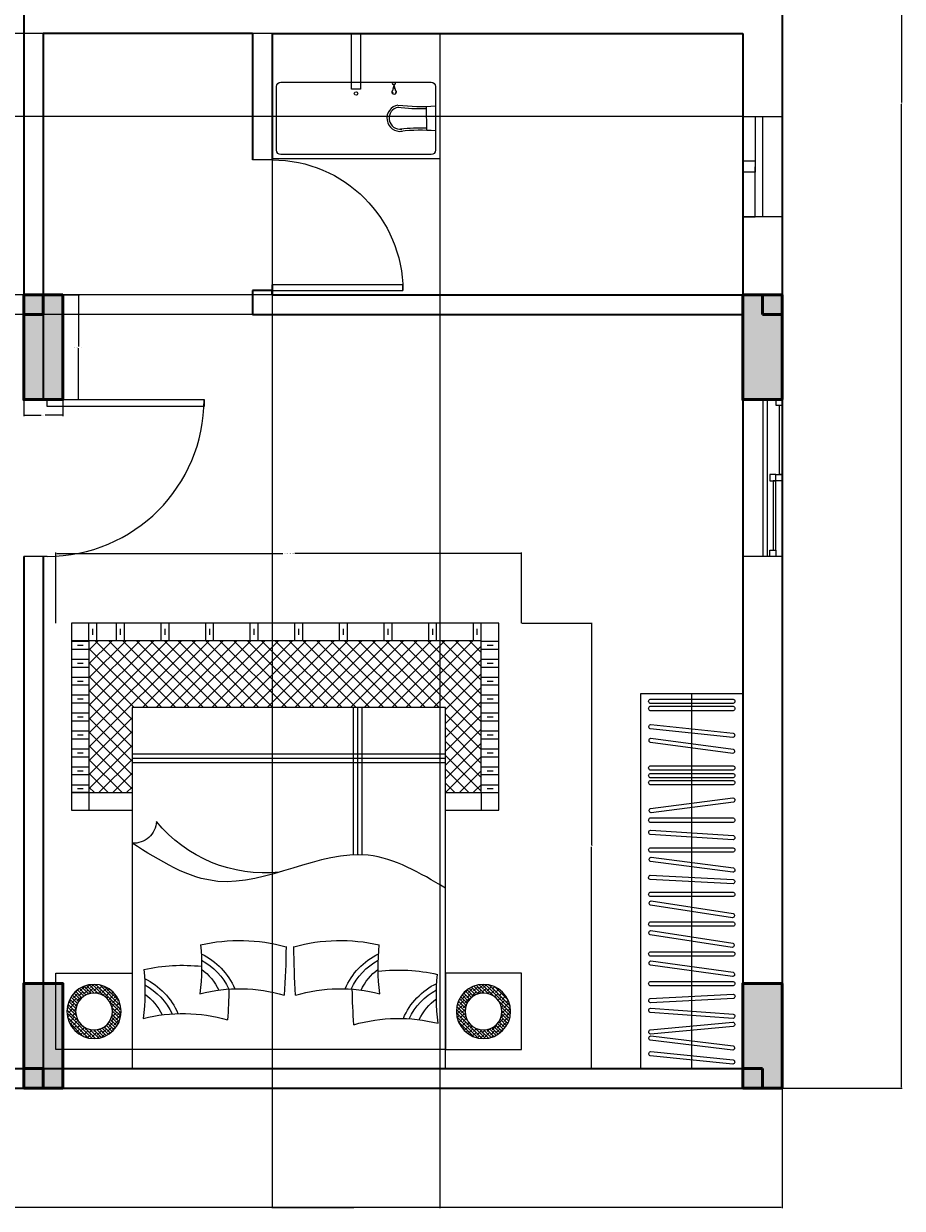
# Model space of a CAD drawing. Units: inches. Extents: x 393 to 993, y 153 to 660.
# Tile 5 of 6: x 791 to 993, y 153 to 425. Entities that reach past the tile are written whole.
import ezdxf

# ---------------------------------------------------------------- set-up
doc = ezdxf.new("R2010")
doc.units = ezdxf.units.IN
doc.header["$MEASUREMENT"] = 0
for name, color, linetype, lineweight in [('A-ANNO-DIMS', 2, 'Continuous', 18), ('A-COLS', 40, 'Continuous', 50), ('A-FLOR-CASE', 72, 'Continuous', 25), ('A-FLOR-FIXT', 9, 'Continuous', 18), ('A-GLAZ', 4, 'Continuous', 20), ('A-WALL', 40, 'Continuous', 35), ('DOORS', 32, 'Continuous', 25), ('FURNITURE', 72, 'Continuous', 18)]:
    doc.layers.add(name, color=color, linetype=linetype, lineweight=lineweight)
doc.styles.get("Standard").update_dxf_attribs({"font": 'arial.ttf'})
doc.dimstyles.get("Standard").update_dxf_attribs({"dimtxt": 0.18, "dimasz": 0.18, "dimexe": 0.18, "dimexo": 0.0625, "dimgap": 0.09, "dimtad": 0, "dimtih": 1, "dimtoh": 1, "dimdec": 1, "dimzin": 0, "dimdsep": 46, "dimlunit": 3, "dimtxsty": 'Standard', "dimcen": 0.09, "dimadec": 0, "dimazin": 0, "dimtfac": 1, "dimtdec": 1, "dimtofl": 0, "dimtmove": 0, "dimatfit": 3, "dimfxl": 1, "dimtolj": 1, "dimtzin": 0, "dimarcsym": 0})

# ---------------------------------------------------------------- blocks, each defined once
blk = doc.blocks.new('*U3')
for p, q in [((0, 0), (0, -6)), ((40, 0), (40, -6))]:
    blk.add_line(p, q)
blk.add_lwpolyline([(0, 0), (0, 40), (1.75, 40), (1.75, 0)], close=True)
blk.add_arc((0, 0), 40, 0, 90)
blk = doc.blocks.new('W')
for p, q in [((518.15, 606.48), (554.15, 606.48)), ((518.15, 605.48), (554.15, 605.48))]:
    blk.add_line(p, q)
for points in [[(518.15, 609.91), (554.15, 609.91), (554.15, 600.91), (518.15, 600.91)], [(519.42, 609.91), (518.15, 609.91), (518.15, 608.51), (519.42, 608.51)], [(519.42, 609.91), (535.35, 609.91), (535.35, 609.3), (519.42, 609.3)], [(535.35, 609.91), (536.78, 609.91), (536.78, 608.51), (535.35, 608.51)], [(536.78, 608.51), (535.35, 608.51), (535.35, 607.12), (536.78, 607.12)], [(552.72, 608.51), (536.78, 608.51), (536.78, 607.91), (552.72, 607.91)], [(552.72, 608.51), (554.15, 608.51), (554.15, 607.12), (552.72, 607.12)]]:
    blk.add_lwpolyline(points, close=True)
blk = doc.blocks.new('MM')
blk.add_line((476.48, 438.96), (476.48, 415.96))
for points in [[(471.98, 438.96), (480.98, 438.96), (480.98, 415.96), (471.98, 415.96), (471.98, 438.96)], [(471.98, 427.46), (471.98, 438.96), (474.84, 438.96), (474.84, 427.46)], [(471.98, 427.46), (471.98, 415.96), (474.84, 415.96), (474.84, 427.46)]]:
    blk.add_lwpolyline(points)
blk.add_lwpolyline([(471.98, 428.78), (474.84, 428.78), (474.84, 426.2), (471.98, 426.2)], close=True)
blk = doc.blocks.new('BED')
h = blk.add_hatch()
h.set_pattern_fill('ANSI38', color=256, scale=4.4)
h.paths.add_polyline_path([(503.33, 587.82, 1), (515.77, 587.82, 1)])
h.paths.add_polyline_path([(513.77, 587.82, -1), (505.33, 587.82, -1)], flags=16)
h = blk.add_hatch()
h.set_pattern_fill('ANSI38', color=256, scale=4.4)
h.paths.add_polyline_path([(592.69, 587.82, 1), (605.13, 587.82, 1)])
h.paths.add_polyline_path([(603.13, 587.82, -1), (594.69, 587.82, -1)], flags=16)
h = blk.add_hatch()
h.set_pattern_fill('ANSI37', color=256, scale=18)
h.paths.add_polyline_path([(518.29, 518.09), (518.29, 537.6), (508.38, 537.6), (508.38, 502.74), (598.4, 502.74), (598.4, 537.6), (590.17, 537.6), (590.17, 518.09)])
for p, q in [((569.1, 551.87), (569.1, 518.09)), ((570.1, 551.87), (570.1, 518.09)), ((571.1, 551.87), (571.1, 518.09)), ((508.38, 537.6), (508.38, 541.6)), ((598.4, 537.6), (598.4, 541.6)), ((508.38, 537.6), (504.38, 537.6)), ((504.38, 537.6), (508.38, 537.6)), ((504.38, 535.78), (508.38, 535.78)), ((505.75, 536.69), (507.09, 536.69)), ((598.4, 537.6), (602.4, 537.6)), ((598.4, 535.78), (602.4, 535.78)), ((599.77, 536.69), (601.11, 536.69)), ((504.38, 533.48), (508.38, 533.48)), ((598.4, 533.48), (602.4, 533.48)), ((504.38, 531.66), (508.38, 531.66)), ((505.75, 532.57), (507.09, 532.57)), ((518.29, 530.67), (590.17, 530.67)), ((598.4, 531.66), (602.4, 531.66)), ((599.77, 532.57), (601.11, 532.57)), ((504.38, 529.37), (508.38, 529.37)), ((504.38, 527.54), (508.38, 527.54)), ((505.75, 528.46), (507.09, 528.46)), ((518.29, 529.67), (590.17, 529.67)), ((518.29, 528.67), (590.17, 528.67)), ((598.4, 529.37), (602.4, 529.37)), ((598.4, 527.54), (602.4, 527.54)), ((599.77, 528.46), (601.11, 528.46)), ((504.38, 525.25), (508.38, 525.25)), ((598.4, 525.25), (602.4, 525.25)), ((504.38, 523.43), (508.38, 523.43)), ((505.75, 524.34), (507.09, 524.34)), ((598.4, 523.43), (602.4, 523.43)), ((599.77, 524.34), (601.11, 524.34)), ((504.38, 521.13), (508.38, 521.13)), ((504.38, 519.31), (508.38, 519.31)), ((505.75, 520.22), (507.09, 520.22)), ((598.4, 521.13), (602.4, 521.13)), ((598.4, 519.31), (602.4, 519.31)), ((599.77, 520.22), (601.11, 520.22)), ((504.38, 517.02), (508.38, 517.02)), ((598.4, 517.02), (602.4, 517.02)), ((504.38, 515.19), (508.38, 515.19)), ((505.75, 516.11), (507.09, 516.11)), ((598.4, 515.19), (602.4, 515.19)), ((599.77, 516.11), (601.11, 516.11)), ((504.38, 512.9), (508.38, 512.9)), ((504.38, 511.08), (508.38, 511.08)), ((505.75, 511.99), (507.09, 511.99)), ((598.4, 512.9), (602.4, 512.9)), ((598.4, 511.08), (602.4, 511.08)), ((599.77, 511.99), (601.11, 511.99)), ((504.38, 508.78), (508.38, 508.78)), ((598.4, 508.78), (602.4, 508.78)), ((504.38, 506.96), (508.38, 506.96)), ((505.75, 507.87), (507.09, 507.87)), ((598.4, 506.96), (602.4, 506.96)), ((599.77, 507.87), (601.11, 507.87)), ((504.38, 504.67), (508.38, 504.67)), ((505.75, 503.76), (507.09, 503.76)), ((598.4, 504.67), (602.4, 504.67)), ((599.77, 503.76), (601.11, 503.76)), ((504.38, 502.84), (508.38, 502.84)), ((508.38, 502.74), (504.38, 502.74)), ((508.38, 502.74), (508.38, 498.74)), ((509.29, 501.37), (509.29, 500.03)), ((510.2, 502.74), (510.2, 498.74)), ((514.7, 502.74), (514.7, 498.74)), ((515.61, 501.37), (515.61, 500.03)), ((516.52, 502.74), (516.52, 498.74)), ((524.93, 502.74), (524.93, 498.74)), ((525.84, 501.37), (525.84, 500.03)), ((526.76, 502.74), (526.76, 498.74)), ((535.17, 502.74), (535.17, 498.74)), ((536.08, 501.37), (536.08, 500.03)), ((536.99, 502.74), (536.99, 498.74)), ((545.4, 502.74), (545.4, 498.74)), ((546.31, 501.37), (546.31, 500.03)), ((547.22, 502.74), (547.22, 498.74)), ((555.64, 502.74), (555.64, 498.74)), ((556.55, 501.37), (556.55, 500.03)), ((557.46, 502.74), (557.46, 498.74)), ((565.87, 502.74), (565.87, 498.74)), ((566.78, 501.37), (566.78, 500.03)), ((567.69, 502.74), (567.69, 498.74)), ((576.11, 502.74), (576.11, 498.74)), ((577.02, 501.37), (577.02, 500.03)), ((577.93, 502.74), (577.93, 498.74)), ((586.34, 502.74), (586.34, 498.74)), ((587.25, 501.37), (587.25, 500.03)), ((588.16, 502.74), (588.16, 498.74)), ((596.58, 502.74), (596.58, 498.74)), ((597.49, 501.37), (597.49, 500.03)), ((598.4, 502.84), (602.4, 502.84)), ((598.4, 502.74), (598.4, 498.74))]:
    blk.add_line(p, q)
for points in [[(518.29, 600.91), (590.17, 600.91), (590.17, 518.09), (518.29, 518.09)], [(518.29, 600.91), (590.17, 600.91), (590.17, 596.58), (518.29, 596.58)], [(518.29, 596.58), (500.81, 596.58), (500.81, 579.05), (518.29, 579.05)], [(590.17, 596.58), (607.65, 596.58), (607.65, 579.05), (590.17, 579.05)]]:
    blk.add_lwpolyline(points, close=True)
for points in [[(590.17, 541.6), (602.4, 541.6), (602.4, 498.74), (504.38, 498.74), (504.38, 541.6), (518.29, 541.6)], [(590.17, 537.6), (598.4, 537.6), (598.4, 502.74), (508.38, 502.74), (508.38, 537.6), (518.29, 537.6)]]:
    blk.add_lwpolyline(points)
for centre, radius in [((509.55, 587.82), 6.22), ((598.91, 587.82), 6.22), ((509.55, 587.82), 4.22), ((598.91, 587.82), 4.22)]:
    blk.add_circle(centre, radius)
for centre, radius, start, end in [((754.03, 578.68), 185.28, 176.2314, 178.7587), ((579.42, 625.84), 36.45, 253.6451, 284.4084), ((639.07, 584.32), 50.97, 172.9945, 185.6503), ((529.91, 624.74), 36.45, 255.5916, 286.3549), ((470.26, 583.22), 50.97, 354.3497, 7.0055), ((514.22, 594.55), 15.87, 295.8431, 336.8331), ((514.22, 594.55), 14.59, 298.6055, 334.9463), ((513.58, 594.12), 12.82, 306.5787, 334.5162), ((355.3, 577.59), 185.28, 1.5729, 3.7686), ((595.11, 595.65), 15.87, 203.1669, 244.1569), ((595.11, 595.65), 14.59, 205.0537, 241.3945), ((595.75, 595.21), 12.82, 205.4838, 233.4213), ((542.93, 619.04), 36.45, 255.5916, 286.3549), ((483.27, 577.52), 50.97, 354.3497, 7.0055), ((527.24, 588.86), 15.87, 295.8431, 336.8331), ((527.24, 588.86), 14.59, 298.6055, 334.9463), ((526.6, 588.42), 12.82, 306.5787, 334.5162), ((368.32, 571.89), 185.28, 0.3263, 3.7686), ((740.67, 571.89), 185.28, 176.2314, 179.6737), ((566.06, 619.04), 36.45, 253.6451, 284.4084), ((581.75, 588.86), 15.87, 203.1669, 244.1569), ((581.75, 588.86), 14.59, 205.0537, 241.3945), ((582.39, 588.42), 12.82, 205.4838, 233.4213), ((625.71, 577.52), 50.97, 172.9945, 185.6503), ((579.44, 619.11), 40.79, 263.4008, 282.6153), ((529.89, 618.01), 40.79, 257.3847, 276.1312), ((542.91, 612.32), 40.79, 257.3847, 285.1893), ((566.08, 612.32), 40.79, 254.8107, 282.6153), ((548.65, 524.17), 31.85, 83.7477, 141.0207), ((518.63, 543.94), 5.27, 2.9325, 93.7021)]:
    blk.add_arc(centre, radius, start, end)
blk.add_open_spline([(590.17, 559.5), (584.37, 556.05), (568.03, 546.36), (541.55, 563.96), (524.71, 553.27), (518.29, 549.19)], degree=3, knots=[0, 0, 0, 0, 19.259502, 54.250447, 75.777559, 75.777559, 75.777559, 75.777559])
blk = doc.blocks.new('COOB')
blk.add_line((626.78, 600.91), (626.78, 514.86))
blk.add_lwpolyline([(638.48, 600.91), (615.08, 600.91), (615.08, 514.86), (638.48, 514.86)], close=True)
for points in [[(636.21, 599.92), (617.25, 598)], [(617.35, 597.01), (636.31, 598.93)], [(636.17, 596.68), (617.24, 594.42)], [(617.36, 593.43), (636.28, 595.69)], [(636.31, 591.25), (617.34, 593.04)], [(617.24, 592.05), (636.21, 590.25)], [(636.24, 589.41), (617.23, 588.06)], [(617.31, 587.07), (636.32, 588.41)], [(617.26, 584.82), (636.29, 583.84)], [(636.35, 584.83), (617.32, 585.82)], [(636.31, 581.92), (617.25, 581.92)], [(617.25, 580.92), (636.31, 580.92)], [(636.15, 579.82), (617.28, 577.19)], [(617.41, 576.2), (636.29, 578.83)], [(636.31, 575.1), (617.25, 575.1)], [(617.25, 574.1), (636.31, 574.1)], [(636.04, 573.13), (617.21, 570.23)], [(617.36, 569.24), (636.2, 572.14)], [(636.31, 568.28), (617.25, 568.28)], [(617.25, 567.28), (636.31, 567.28)], [(636.12, 566.32), (617.28, 563.41)], [(617.44, 562.42), (636.27, 565.34)], [(636.31, 561.46), (617.25, 561.46)], [(617.25, 560.46), (636.31, 560.46)], [(636.25, 558.53), (617.21, 557.57)], [(617.26, 556.57), (636.3, 557.54)], [(636.23, 555.87), (617.33, 553.42)], [(617.46, 552.43), (636.36, 554.88)], [(636.31, 551.24), (617.25, 551.24)], [(617.25, 550.24), (636.31, 550.24)], [(636.26, 548.43), (617.24, 547.23)], [(617.3, 546.23), (636.32, 547.43)], [(636.31, 544.42), (617.25, 544.42)], [(617.25, 543.42), (636.31, 543.42)], [(617.33, 541.23), (636.23, 538.78)], [(636.36, 539.77), (617.46, 542.23)], [(636.31, 535.8), (617.25, 535.8)], [(617.25, 534.8), (636.31, 534.8)], [(636.31, 534.19), (617.25, 534.19)], [(617.25, 533.19), (636.31, 533.19)], [(636.31, 532.44), (617.25, 532.44)], [(617.25, 531.44), (636.31, 531.44)], [(636.16, 528.62), (617.27, 526.12)], [(617.4, 525.13), (636.29, 527.62)], [(636.19, 524.96), (617.24, 522.96)], [(617.35, 521.97), (636.3, 523.96)], [(636.31, 518.8), (617.25, 518.8)], [(617.25, 517.8), (636.31, 517.8)], [(636.31, 517.14), (617.25, 517.14)], [(617.25, 516.14), (636.31, 516.14)]]:
    blk.add_lwpolyline(points)
for centre, start, end in [((636.11, 599.41), 291.987, 79.5876), ((617.44, 597.52), 111.987, 259.5876), ((636.08, 596.17), 293.0233, 80.6239), ((617.43, 592.53), 100.7874, 248.388), ((617.45, 593.94), 113.0233, 260.6239), ((636.12, 590.76), 280.7874, 68.388), ((617.41, 587.58), 110.2473, 257.8479), ((636.13, 588.9), 290.2473, 77.8479), ((617.43, 585.31), 103.2278, 250.8284), ((636.18, 584.34), 283.2278, 70.8284), ((617.4, 581.42), 106.1997, 253.8003), ((636.16, 581.42), 286.1997, 73.8003), ((636.08, 579.31), 294.1332, 81.7338), ((617.49, 576.72), 114.1332, 261.7338), ((617.4, 574.6), 106.1997, 253.8003), ((636.16, 574.6), 286.1997, 73.8003), ((635.98, 572.61), 294.9436, 82.5442), ((617.4, 567.78), 106.1997, 253.8003), ((617.43, 569.76), 114.9436, 262.5442), ((636.16, 567.78), 286.1997, 73.8003), ((636.05, 565.81), 294.9996, 82.6002), ((617.5, 562.94), 114.9996, 262.6002), ((617.4, 560.96), 106.1997, 253.8003), ((636.16, 560.96), 286.1997, 73.8003), ((617.38, 557.08), 109.0898, 256.6904), ((636.13, 558.03), 289.0898, 76.6904), ((636.15, 555.36), 293.5955, 81.1961), ((617.54, 552.94), 113.5955, 261.1961), ((617.4, 550.74), 106.1997, 253.8003), ((636.16, 550.74), 286.1997, 73.8003), ((617.41, 546.74), 109.8088, 257.4094), ((636.14, 547.92), 289.8088, 77.4094), ((617.4, 543.92), 106.1997, 253.8003), ((636.16, 543.92), 286.1997, 73.8003), ((617.54, 541.71), 98.8065, 246.4071), ((636.15, 539.3), 278.8065, 66.4071), ((617.4, 535.3), 106.1997, 253.8003), ((636.16, 535.3), 286.1997, 73.8003), ((617.4, 533.69), 106.1997, 253.8003), ((636.16, 533.69), 286.1997, 73.8003), ((617.4, 531.94), 106.1997, 253.8003), ((636.16, 531.94), 286.1997, 73.8003), ((636.08, 528.1), 293.7284, 81.329), ((617.48, 525.64), 113.7284, 261.329), ((636.1, 524.44), 292.2058, 79.8064), ((617.44, 522.48), 112.2058, 259.8064), ((617.4, 518.3), 106.1997, 253.8003), ((617.4, 516.64), 106.1997, 253.8003), ((636.16, 518.3), 286.1997, 73.8003), ((636.16, 516.64), 286.1997, 73.8003)]:
    blk.add_arc(centre, 0.521, start, end)
blk = doc.blocks.new('COL-9X24-RH')
h = blk.add_hatch(color=256)
h.dxf.hatch_style = 1
h.paths.add_polyline_path([(4.5, 19.5), (4.5, 24), (0, 24), (0, 0), (9, 0), (9, 19.5)])
h = blk.add_hatch(color=256)
h.dxf.hatch_style = 1
h.paths.add_polyline_path([(4.5, 19.5), (9, 19.5), (9, 24), (4.5, 24)])
for p, q in [((4.5, 24), (4.5, 19.5)), ((4.5, 24), (9, 24)), ((9, 24), (9, 19.5)), ((4.5, 19.5), (9, 19.5))]:
    blk.add_line(p, q)
blk.add_lwpolyline([(0, 24), (9, 24), (9, 0), (0, 0), (0, 24)])
blk = doc.blocks.new('COL-9X24-LH')
h = blk.add_hatch(color=256)
h.dxf.hatch_style = 1
h.paths.add_polyline_path([(4.5, 24), (0, 24), (0, 19.5), (4.5, 19.5)])
h = blk.add_hatch(color=256)
h.dxf.hatch_style = 1
h.paths.add_polyline_path([(4.5, 19.5), (0, 19.5), (0, 0), (9, 0), (9, 24), (4.5, 24)])
for p, q in [((4.5, 24), (0, 24)), ((0, 24), (0, 19.5)), ((4.5, 24), (4.5, 19.5)), ((4.5, 19.5), (0, 19.5))]:
    blk.add_line(p, q)
blk.add_lwpolyline([(9, 24), (0, 24), (0, 0), (9, 0), (9, 24)])
blk = doc.blocks.new('*D20')
at = {"layer": 'A-ANNO-DIMS', "color": 0, "lineweight": -2, "transparency": 16777216}
for p, q in [((800.54, 362.91), (804.26, 362.91)), ((804.08, 362.73), (804.08, 351.09)), ((804.08, 339.09), (804.08, 350.72)), ((800.54, 338.91), (804.26, 338.91))]:
    blk.add_line(p, q, dxfattribs=at)
at = {"layer": 'A-ANNO-DIMS', "color": 0, "transparency": 16777216}
for points in [[(804.05, 362.73), (804.11, 362.73), (804.08, 362.91)], [(804.05, 339.09), (804.11, 339.09), (804.08, 338.91)]]:
    blk.add_solid(points, dxfattribs=at)
at = {"layer": 'Defpoints', "color": 0, "transparency": 16777216}
for p in [(800.48, 362.91), (804.08, 362.91), (800.48, 338.91)]:
    blk.add_point(p, dxfattribs=at)
at = {"layer": 'A-ANNO-DIMS', "color": 0, "transparency": 16777216, "insert": (804.08, 350.91), "char_height": 0.18, "attachment_point": 5}
blk.add_mtext('\\A1;LH COL. 24 TYP.', dxfattribs=at)
blk = doc.blocks.new('*D21')
at = {"layer": 'A-ANNO-DIMS', "color": 0, "lineweight": -2, "transparency": 16777216}
for p, q in [((791.48, 338.84), (791.48, 335.13)), ((800.48, 338.84), (800.48, 335.13)), ((791.66, 335.31), (795.52, 335.31)), ((800.3, 335.31), (796.44, 335.31))]:
    blk.add_line(p, q, dxfattribs=at)
at = {"layer": 'A-ANNO-DIMS', "color": 0, "transparency": 16777216}
for points in [[(791.66, 335.34), (791.66, 335.28), (791.48, 335.31)], [(800.3, 335.34), (800.3, 335.28), (800.48, 335.31)]]:
    blk.add_solid(points, dxfattribs=at)
at = {"layer": 'Defpoints', "color": 0, "transparency": 16777216}
for p in [(791.48, 338.91), (800.48, 338.91), (800.48, 335.31)]:
    blk.add_point(p, dxfattribs=at)
at = {"layer": 'A-ANNO-DIMS', "color": 0, "transparency": 16777216, "insert": (795.98, 335.31), "char_height": 0.18, "attachment_point": 5}
blk.add_mtext('\\A1;9 TYP.', dxfattribs=at)
blk = doc.blocks.new('*D32')
at = {"layer": 'A-ANNO-DIMS', "color": 0, "lineweight": -2, "transparency": 16777216}
for p, q in [((798.88, 287.63), (798.88, 303.78)), ((799.06, 303.6), (850.92, 303.6)), ((905.55, 303.6), (853.69, 303.6)), ((905.73, 287.63), (905.73, 303.78))]:
    blk.add_line(p, q, dxfattribs=at)
at = {"layer": 'A-ANNO-DIMS', "color": 0, "transparency": 16777216}
for points in [[(799.06, 303.63), (799.06, 303.57), (798.88, 303.6)], [(905.55, 303.63), (905.55, 303.57), (905.73, 303.6)]]:
    blk.add_solid(points, dxfattribs=at)
at = {"layer": 'Defpoints', "color": 0, "transparency": 16777216}
for p in [(905.73, 303.6), (798.88, 287.57), (905.73, 287.57)]:
    blk.add_point(p, dxfattribs=at)
at = {"layer": 'A-ANNO-DIMS', "color": 0, "transparency": 16777216, "insert": (852.3, 303.6), "char_height": 0.18, "attachment_point": 5}
blk.add_mtext('\\A1;BED GROUP 107 TYP.', dxfattribs=at)
blk = doc.blocks.new('*D33')
at = {"layer": 'A-ANNO-DIMS', "color": 0, "lineweight": -2, "transparency": 16777216}
for p, q in [((905.79, 287.57), (921.93, 287.57)), ((921.75, 287.39), (921.75, 236.67)), ((921.75, 185.59), (921.75, 236.31)), ((905.79, 185.41), (921.93, 185.41))]:
    blk.add_line(p, q, dxfattribs=at)
at = {"layer": 'A-ANNO-DIMS', "color": 0, "transparency": 16777216}
for points in [[(921.72, 287.39), (921.78, 287.39), (921.75, 287.57)], [(921.72, 185.59), (921.78, 185.59), (921.75, 185.41)]]:
    blk.add_solid(points, dxfattribs=at)
at = {"layer": 'Defpoints', "color": 0, "transparency": 16777216}
for p in [(905.73, 287.57), (905.73, 185.41), (921.75, 185.41)]:
    blk.add_point(p, dxfattribs=at)
at = {"layer": 'A-ANNO-DIMS', "color": 0, "transparency": 16777216, "insert": (921.75, 236.49), "char_height": 0.18, "attachment_point": 5}
blk.add_mtext('\\A1;102 TYP.', dxfattribs=at)
blk = doc.blocks.new('*D44')
at = {"layer": 'A-ANNO-DIMS', "color": 0, "lineweight": -2, "transparency": 16777216}
for p, q in [((471.98, 180.84), (471.98, 153.33)), ((965.48, 180.84), (965.48, 153.33)), ((472.16, 153.51), (718.33, 153.51)), ((965.3, 153.51), (719.13, 153.51))]:
    blk.add_line(p, q, dxfattribs=at)
at = {"layer": 'A-ANNO-DIMS', "color": 0, "transparency": 16777216}
for points in [[(472.16, 153.54), (472.16, 153.48), (471.98, 153.51)], [(965.3, 153.54), (965.3, 153.48), (965.48, 153.51)]]:
    blk.add_solid(points, dxfattribs=at)
at = {"layer": 'Defpoints', "color": 0, "transparency": 16777216}
for p in [(471.98, 180.91), (965.48, 180.91), (965.48, 153.51)]:
    blk.add_point(p, dxfattribs=at)
at = {"layer": 'A-ANNO-DIMS', "color": 0, "transparency": 16777216, "insert": (718.73, 153.51), "char_height": 0.18, "attachment_point": 5}
blk.add_mtext('\\A1;493.5', dxfattribs=at)
blk = doc.blocks.new('*D45')
at = {"layer": 'A-ANNO-DIMS', "color": 0, "lineweight": -2, "transparency": 16777216}
for p, q in [((796.04, 632.91), (993.06, 632.91)), ((992.88, 632.73), (992.88, 407.09)), ((992.88, 181.09), (992.88, 406.72)), ((965.54, 180.91), (993.06, 180.91))]:
    blk.add_line(p, q, dxfattribs=at)
at = {"layer": 'A-ANNO-DIMS', "color": 0, "transparency": 16777216}
for points in [[(992.85, 632.73), (992.91, 632.73), (992.88, 632.91)], [(992.85, 181.09), (992.91, 181.09), (992.88, 180.91)]]:
    blk.add_solid(points, dxfattribs=at)
at = {"layer": 'Defpoints', "color": 0, "transparency": 16777216}
for p in [(795.98, 632.91), (992.88, 632.91), (965.48, 180.91)]:
    blk.add_point(p, dxfattribs=at)
at = {"layer": 'A-ANNO-DIMS', "color": 0, "transparency": 16777216, "insert": (992.88, 406.91), "char_height": 0.18, "attachment_point": 5}
blk.add_mtext('\\A1;452', dxfattribs=at)
blk = doc.blocks.new('*D62')
at = {"layer": 'A-ANNO-DIMS', "color": 0, "lineweight": -2, "transparency": 16777216}
for p, q in [((848.42, 422.91), (393.4, 422.91)), ((393.58, 422.73), (393.58, 393.09)), ((393.58, 363.09), (393.58, 392.72)), ((848.42, 362.91), (393.4, 362.91))]:
    blk.add_line(p, q, dxfattribs=at)
at = {"layer": 'A-ANNO-DIMS', "color": 0, "transparency": 16777216}
for points in [[(393.55, 422.73), (393.61, 422.73), (393.58, 422.91)], [(393.55, 363.09), (393.61, 363.09), (393.58, 362.91)]]:
    blk.add_solid(points, dxfattribs=at)
at = {"layer": 'Defpoints', "color": 0, "transparency": 16777216}
for p in [(393.58, 422.91), (848.48, 422.91), (848.48, 362.91)]:
    blk.add_point(p, dxfattribs=at)
at = {"layer": 'A-ANNO-DIMS', "color": 0, "transparency": 16777216, "insert": (393.58, 392.91), "char_height": 0.18, "attachment_point": 5}
blk.add_mtext('\\A1;60', dxfattribs=at)
blk = doc.blocks.new('*D70')
at = {"layer": 'A-ANNO-DIMS', "color": 0, "lineweight": -2, "transparency": 16777216}
for p, q in [((848.48, 393.84), (848.48, 153.33)), ((886.99, 394.05), (886.99, 153.33)), ((848.66, 153.51), (867.27, 153.51)), ((886.81, 153.51), (868.2, 153.51))]:
    blk.add_line(p, q, dxfattribs=at)
at = {"layer": 'A-ANNO-DIMS', "color": 0, "transparency": 16777216}
for points in [[(848.66, 153.54), (848.66, 153.48), (848.48, 153.51)], [(886.81, 153.54), (886.81, 153.48), (886.99, 153.51)]]:
    blk.add_solid(points, dxfattribs=at)
at = {"layer": 'Defpoints', "color": 0, "transparency": 16777216}
for p in [(848.48, 393.91), (886.99, 394.11), (886.99, 153.51)]:
    blk.add_point(p, dxfattribs=at)
at = {"layer": 'A-ANNO-DIMS', "color": 0, "transparency": 16777216, "insert": (867.74, 153.51), "char_height": 0.18, "attachment_point": 5}
blk.add_mtext('\\A1;38.515', dxfattribs=at)
blk = doc.blocks.new('*D71')
at = {"layer": 'A-ANNO-DIMS', "color": 0, "lineweight": -2, "transparency": 16777216}
for p, q in [((956.42, 358.41), (393.4, 358.41)), ((393.58, 358.23), (393.58, 272.09)), ((393.58, 185.59), (393.58, 271.72)), ((956.42, 185.41), (393.4, 185.41))]:
    blk.add_line(p, q, dxfattribs=at)
at = {"layer": 'A-ANNO-DIMS', "color": 0, "transparency": 16777216}
for points in [[(393.55, 358.23), (393.61, 358.23), (393.58, 358.41)], [(393.55, 185.59), (393.61, 185.59), (393.58, 185.41)]]:
    blk.add_solid(points, dxfattribs=at)
at = {"layer": 'Defpoints', "color": 0, "transparency": 16777216}
for p in [(393.58, 358.41), (956.48, 358.41), (956.48, 185.41)]:
    blk.add_point(p, dxfattribs=at)
at = {"layer": 'A-ANNO-DIMS', "color": 0, "transparency": 16777216, "insert": (393.58, 271.91), "char_height": 0.18, "attachment_point": 5}
blk.add_mtext('\\A1;173', dxfattribs=at)
blk = doc.blocks.new('*D73')
at = {"layer": 'A-ANNO-DIMS', "color": 0, "lineweight": -2, "transparency": 16777216}
for p, q in [((956.42, 422.91), (393.4, 422.91)), ((393.58, 422.73), (393.58, 413.55)), ((393.58, 404.01), (393.58, 413.19)), ((956.42, 403.83), (393.4, 403.83))]:
    blk.add_line(p, q, dxfattribs=at)
at = {"layer": 'A-ANNO-DIMS', "color": 0, "transparency": 16777216}
for points in [[(393.55, 422.73), (393.61, 422.73), (393.58, 422.91)], [(393.55, 404.01), (393.61, 404.01), (393.58, 403.83)]]:
    blk.add_solid(points, dxfattribs=at)
at = {"layer": 'Defpoints', "color": 0, "transparency": 16777216}
for p in [(393.58, 422.91), (956.48, 422.91), (956.48, 403.83)]:
    blk.add_point(p, dxfattribs=at)
at = {"layer": 'A-ANNO-DIMS', "color": 0, "transparency": 16777216, "insert": (393.58, 413.37), "char_height": 0.18, "attachment_point": 5}
blk.add_mtext('\\A1;19.08', dxfattribs=at)

msp = doc.modelspace()

# ---------------------------------------------------------------- linework, layer by layer
at = {"layer": 'A-FLOR-FIXT'}
for p, q in [((876.4343, 411.1507), (876.0988, 409.7881)), ((876.4343, 411.1507), (876.7697, 409.7881)), ((883.8547, 406.1773), (883.9259, 400.6756))]:
    msp.add_line(p, q, dxfattribs=at)
for points in [[(848.4798, 422.9066), (886.9946, 422.9066), (886.9946, 394.1107), (848.4798, 394.1107)], [(866.7175, 422.9066), (868.757, 422.9066), (868.757, 410.1212), (866.7175, 410.1212)]]:
    msp.add_lwpolyline(points, close=True, dxfattribs=at)
msp.add_lwpolyline([(850.4798, 411.7443), (884.9946, 411.7443, -0.41421356), (885.9946, 410.7443), (885.9946, 396.1107, -0.41421356), (884.9946, 395.1107), (850.4798, 395.1107, -0.41421356), (849.4798, 396.1107), (849.4798, 410.7443, -0.41421356)], format="xyb", close=True, dxfattribs=at)
for centre, radius in [((876.4343, 411.4475), 0.2968), ((867.7372, 409.1309), 0.3984)]:
    msp.add_circle(centre, radius, dxfattribs=at)
for centre, radius, start, end in [((876.1946, 409.5516), 0.2552, 112.042136, 283.977865), ((876.4889, 409.5089), 0.5382, 183.860703, 3.860703), ((876.0602, 409.2186), 0.2138, 23.529492, 112.520144), ((876.4347, 410.0747), 0.2624, 25.697196, 155.199338), ((876.7873, 409.5501), 0.2386, 263.396554, 94.209702), ((876.9378, 409.2529), 0.1879, 72.401892, 161.302932), ((877.8525, 403.4832), 3.0395, 99.22759, 278.823113), ((877.8525, 403.4832), 2.5395, 99.22759, 278.823113), ((882.5946, 448.4081), 42.7497, 262.889885, 271.642526), ((882.5946, 448.4081), 42.2497, 262.889885, 274.615828), ((882.5946, 448.4081), 42.7497, 274.561726, 274.615828), ((882.5946, 358.4469), 42.7497, 88.224166, 96.213079), ((882.5946, 358.4469), 42.2497, 85.384172, 96.213079), ((882.5946, 358.4469), 42.7497, 85.384172, 85.438274)]:
    msp.add_arc(centre, radius, start, end, dxfattribs=at)
at = {"layer": 'A-WALL'}
for p, q in [((965.4798, 609.9066), (965.4798, 180.9066)), ((791.4798, 427.4066), (791.4798, 362.9066)), ((843.9798, 422.9066), (795.9798, 422.9066)), ((795.9798, 422.9066), (795.9798, 338.9066)), ((843.9798, 422.9066), (843.9798, 393.9066)), ((848.4798, 422.9066), (956.4798, 422.9066)), ((848.4798, 422.9066), (848.4798, 393.9066)), ((956.4798, 422.9066), (956.4798, 362.9066)), ((848.4798, 365.2191), (848.4798, 362.9066)), ((848.4798, 363.9066), (843.9798, 363.9066)), ((843.9798, 363.9066), (843.9798, 358.4066)), ((848.4798, 362.9066), (848.4798, 363.9066)), ((848.4798, 362.9066), (956.4798, 362.9066)), ((843.9798, 358.4066), (956.4798, 358.4066)), ((956.4798, 358.4066), (956.4798, 185.4066)), ((791.4798, 302.9066), (791.4798, 180.9066)), ((795.9798, 302.9066), (795.9798, 180.9066)), ((687.4798, 185.4066), (956.4798, 185.4066)), ((687.4798, 180.9066), (965.4798, 180.9066))]:
    msp.add_line(p, q, dxfattribs=at)

# ---------------------------------------------------------------- block references
at = {"layer": 'A-COLS'}
for name, p in [('COL-9X24-LH', (791.48, 338.907)), ('COL-9X24-RH', (956.48, 338.907))]:
    msp.add_blockref(name, p, dxfattribs=at)
at = {"layer": 'A-COLS', "rotation": 180}
for p in [(800.4796, 204.9063), (965.4796, 204.9063)]:
    msp.add_blockref('COL-9X24-RH', p, dxfattribs=at)
at = {"layer": 'A-FLOR-CASE', "xscale": -1, "rotation": 180}
msp.add_blockref('COOB', (318, 786.3133), dxfattribs=at)
at = {"layer": 'A-GLAZ'}
msp.add_blockref('MM', (484.5, -35.1283), dxfattribs=at)
at = {"layer": 'A-GLAZ', "rotation": 270}
msp.add_blockref('W', (355.5732, 857.0554), dxfattribs=at)
at = {"layer": 'DOORS'}
for p, xscale, yscale, zscale, rotation in [((848.4798, 363.9066), -0.75, 0.75, 0.75, 269.9999999999997), ((796.8798, 338.9066), 0.9, 0.9, 0.9, 270.0000000000003)]:
    msp.add_blockref('*U3', p, dxfattribs=dict(at, xscale=xscale, yscale=yscale, zscale=zscale, rotation=rotation))
at = {"layer": 'FURNITURE', "xscale": -1, "rotation": 180}
msp.add_blockref('BED', (298.074, 786.3133), dxfattribs=at)

# ---------------------------------------------------------------- dimensions: what is measured, and where the dimension line sits
at = {"layer": 'A-ANNO-DIMS'}
for base, p1, p2, override, picture, middle in [((992.8798, 632.9066), (965.4798, 180.9066), (795.9798, 632.9066), {"dimdec": 0, "dimlfac": 1, "dimrnd": 0, "dimzin": 0, "dimdsep": 46, "dimlunit": 2}, '*D45', (992.8798, 406.9066)), ((393.5798, 422.9066), (956.4798, 403.8282), (956.4798, 422.9066), {"dimdec": 2, "dimlfac": 1, "dimrnd": 0, "dimzin": 0, "dimdsep": 46, "dimlunit": 2}, '*D73', (393.5798, 413.3674)), ((393.5798, 422.9066), (848.4798, 362.9066), (848.4798, 422.9066), {"dimdec": 0, "dimlfac": 1, "dimrnd": 0, "dimzin": 0, "dimdsep": 46, "dimlunit": 2}, '*D62', (393.5798, 392.9066)), ((393.5798, 358.4066), (956.4798, 185.4066), (956.4798, 358.4066), {"dimdec": 0, "dimlfac": 1, "dimrnd": 0, "dimzin": 0, "dimdsep": 46, "dimlunit": 2}, '*D71', (393.5798, 271.9066))]:
    dim = msp.add_linear_dim(base=base, p1=p1, p2=p2, angle=90, dimstyle='Standard', override=override, dxfattribs=at)
    dim.commit()
    dim.dimension.update_dxf_attribs({"geometry": picture, "text_midpoint": middle})
for base, p1, p2, override, picture, middle in [((886.9946, 153.5066), (848.4798, 393.9066), (886.9946, 394.1107), {"dimdec": 3, "dimlfac": 1, "dimrnd": 0, "dimzin": 0, "dimdsep": 46, "dimlunit": 2}, '*D70', (867.7372, 153.5066)), ((965.4798, 153.5066), (471.9798, 180.9066), (965.4798, 180.9066), {"dimdec": 1, "dimlfac": 1, "dimrnd": 0, "dimzin": 0, "dimdsep": 46, "dimlunit": 2}, '*D44', (718.7298, 153.5066))]:
    dim = msp.add_linear_dim(base=base, p1=p1, p2=p2, dimstyle='Standard', override=override, dxfattribs=at)
    dim.commit()
    dim.dimension.update_dxf_attribs({"geometry": picture, "text_midpoint": middle})
for base, p1, p2, angle, text, picture, middle in [((804.0798, 362.9066), (800.4798, 338.9066), (800.4798, 362.9066), 90, 'LH COL. <> TYP.', '*D20', (804.0798, 350.9066)), ((921.7515, 185.4066), (905.7252, 287.5689), (905.7252, 185.4066), 270, '<> TYP.', '*D33', (921.7515, 236.4878))]:
    dim = msp.add_linear_dim(base=base, p1=p1, p2=p2, angle=angle, text=text, dimstyle='Standard', override={"dimdec": 0, "dimlfac": 1, "dimrnd": 0, "dimzin": 0, "dimdsep": 46, "dimlunit": 2}, dxfattribs=at)
    dim.commit()
    dim.dimension.update_dxf_attribs({"geometry": picture, "text_midpoint": middle})
for base, p1, p2, text, picture, middle in [((800.4798, 335.3066), (791.4798, 338.9066), (800.4798, 338.9066), '<> TYP.', '*D21', (795.9798, 335.3066)), ((905.7252, 303.5952), (798.8829, 287.5689), (905.7252, 287.5689), 'BED GROUP <> TYP.', '*D32', (852.304, 303.5952))]:
    dim = msp.add_linear_dim(base=base, p1=p1, p2=p2, text=text, dimstyle='Standard', override={"dimdec": 0, "dimlfac": 1, "dimrnd": 0, "dimzin": 0, "dimdsep": 46, "dimlunit": 2}, dxfattribs=at)
    dim.commit()
    dim.dimension.update_dxf_attribs({"geometry": picture, "text_midpoint": middle})

doc.saveas('drawing.dxf')
